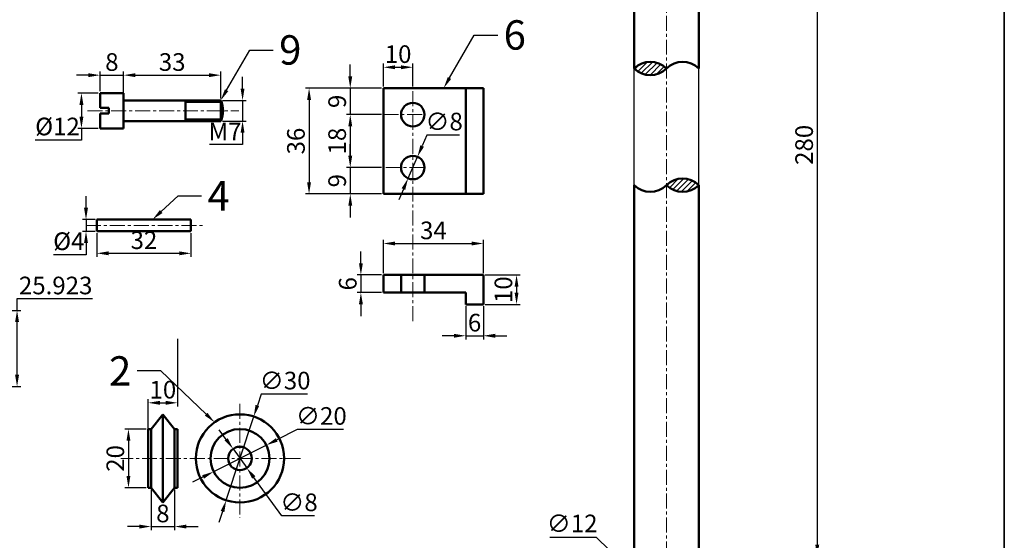
# Model space of a CAD drawing. Units: millimetres. Extents: x 44 to 571, y -292 to 291.
# Tile 3 of 4: x 236 to 571, y -69 to 108. Entities that reach past the tile are written whole.
import ezdxf
from ezdxf import colors
from ezdxf.entities.mleader import LeaderData, LeaderLine
from ezdxf.math import Vec2, Vec3

# ---------------------------------------------------------------- set-up
doc = ezdxf.new("R2010")
doc.units = ezdxf.units.MM
doc.header["$LTSCALE"] = 0.4
doc.linetypes.add('CENTER', pattern=[50.8, 31.75, -6.35, 6.35, -6.35])
for name, color, linetype, lineweight in [('M-CNTR', 1, 'CENTER', 18), ('M-DIMS', 2, 'Continuous', 25), ('M-HATC', 8, 'Continuous', 18), ('M-OUTL', 7, 'Continuous', 50), ('M-TEXT', 3, 'Continuous', 25), ('M-TTLB', 7, 'Continuous', 35)]:
    doc.layers.add(name, color=color, linetype=linetype, lineweight=lineweight)
doc.styles.get("Standard").update_dxf_attribs({"font": 'arial.ttf'})
doc.dimstyles.new('ISO-25', dxfattribs={"dimtxt": 6, "dimasz": 4, "dimexe": 1.25, "dimexo": 0.625, "dimtad": 1, "dimtoh": 1, "dimdec": 0, "dimtxsty": 'Standard', "dimcen": 2.5, "dimadec": 0, "dimazin": 0, "dimtfac": 1, "dimtdec": 0, "dimtmove": 0, "dimatfit": 3, "dimfxl": 1, "dimarcsym": 0})

# ---------------------------------------------------------------- blocks, each defined once
blk = doc.blocks.new('*D37')
at = {"layer": 'Defpoints', "color": 0, "ltscale": 0.4, "transparency": 16777216}
for p in [(271.14, 89.1), (263.14, 83), (271.14, 83)]:
    blk.add_point(p, dxfattribs=at)
at = {"layer": 'M-DIMS', "color": 0, "lineweight": -2, "ltscale": 0.4, "transparency": 16777216}
for p, q in [((259.14, 89.1), (255.14, 89.1)), ((263.14, 83.63), (263.14, 90.35)), ((263.14, 89.1), (271.14, 89.1)), ((271.14, 83.63), (271.14, 90.35)), ((275.14, 89.1), (279.14, 89.1))]:
    blk.add_line(p, q, dxfattribs=at)
at = {"layer": 'M-DIMS', "color": 0, "ltscale": 0.4, "transparency": 16777216}
for points in [[(259.14, 89.77), (259.14, 88.44), (263.14, 89.1)], [(275.14, 89.77), (275.14, 88.44), (271.14, 89.1)]]:
    blk.add_solid(points, dxfattribs=at)
at = {"layer": 'M-DIMS', "color": 0, "ltscale": 0.4, "transparency": 16777216, "insert": (267.14, 92.79), "char_height": 6, "attachment_point": 5}
blk.add_mtext('8', dxfattribs=at)
blk = doc.blocks.new('*D38')
at = {"layer": 'Defpoints', "color": 0, "ltscale": 0.4, "transparency": 16777216}
for p in [(304.14, 89.1), (271.14, 80.5), (304.14, 80.5)]:
    blk.add_point(p, dxfattribs=at)
at = {"layer": 'M-DIMS', "color": 0, "lineweight": -2, "ltscale": 0.4, "transparency": 16777216}
for p, q in [((271.14, 81.13), (271.14, 90.35)), ((275.14, 89.1), (300.14, 89.1)), ((304.14, 81.13), (304.14, 90.35))]:
    blk.add_line(p, q, dxfattribs=at)
at = {"layer": 'M-DIMS', "color": 0, "ltscale": 0.4, "transparency": 16777216}
for points in [[(275.14, 89.77), (275.14, 88.44), (271.14, 89.1)], [(300.14, 89.77), (300.14, 88.44), (304.14, 89.1)]]:
    blk.add_solid(points, dxfattribs=at)
at = {"layer": 'M-DIMS', "color": 0, "ltscale": 0.4, "transparency": 16777216, "insert": (287.64, 92.79), "char_height": 6, "attachment_point": 5}
blk.add_mtext('33', dxfattribs=at)
blk = doc.blocks.new('*D39')
at = {"layer": 'Defpoints', "color": 0, "ltscale": 0.4, "transparency": 16777216}
for p in [(304.14, 80.5), (304.14, 73.5), (311.58, 73.5)]:
    blk.add_point(p, dxfattribs=at)
at = {"layer": 'M-DIMS', "color": 0, "lineweight": -2, "ltscale": 0.4, "transparency": 16777216}
for p, q in [((311.58, 84.5), (311.58, 88.5)), ((304.77, 80.5), (312.83, 80.5)), ((311.58, 80.5), (311.58, 73.5)), ((304.77, 73.5), (312.83, 73.5)), ((311.58, 69.5), (311.58, 65.5)), ((311.58, 65.5), (300.31, 65.5))]:
    blk.add_line(p, q, dxfattribs=at)
at = {"layer": 'M-DIMS', "color": 0, "ltscale": 0.4, "transparency": 16777216}
for points in [[(310.91, 84.5), (312.24, 84.5), (311.58, 80.5)], [(310.91, 69.5), (312.24, 69.5), (311.58, 73.5)]]:
    blk.add_solid(points, dxfattribs=at)
at = {"layer": 'M-DIMS', "color": 0, "ltscale": 0.4, "transparency": 16777216, "insert": (305.63, 69.13), "char_height": 6, "attachment_point": 5}
blk.add_mtext('M7', dxfattribs=at)
blk = doc.blocks.new('*D40')
at = {"layer": 'Defpoints', "color": 0, "ltscale": 0.4, "transparency": 16777216}
for p in [(263.14, 83), (256.8, 71), (263.14, 71)]:
    blk.add_point(p, dxfattribs=at)
at = {"layer": 'M-DIMS', "color": 0, "lineweight": -2, "ltscale": 0.4, "transparency": 16777216}
for p, q in [((262.52, 83), (255.55, 83)), ((256.8, 79), (256.8, 75)), ((262.52, 71), (255.55, 71)), ((256.8, 71), (256.8, 67)), ((256.8, 67), (241.11, 67))]:
    blk.add_line(p, q, dxfattribs=at)
at = {"layer": 'M-DIMS', "color": 0, "ltscale": 0.4, "transparency": 16777216}
for points in [[(256.13, 79), (257.47, 79), (256.8, 83)], [(256.13, 75), (257.47, 75), (256.8, 71)]]:
    blk.add_solid(points, dxfattribs=at)
at = {"layer": 'M-DIMS', "color": 0, "ltscale": 0.4, "transparency": 16777216, "insert": (248.65, 70.86), "char_height": 6, "attachment_point": 5}
blk.add_mtext('%%C12', dxfattribs=at)
blk = doc.blocks.new('*D41')
at = {"layer": 'Defpoints', "color": 0, "ltscale": 0.4, "transparency": 16777216}
for p in [(359.46, 21.12), (351.81, 15.12), (359.46, 15.12)]:
    blk.add_point(p, dxfattribs=at)
at = {"layer": 'M-DIMS', "color": 0, "lineweight": -2, "ltscale": 0.4, "transparency": 16777216}
for p, q in [((351.81, 25.12), (351.81, 29.12)), ((358.83, 21.12), (350.56, 21.12)), ((351.81, 21.12), (351.81, 15.12)), ((358.83, 15.12), (350.56, 15.12)), ((351.81, 11.12), (351.81, 7.12))]:
    blk.add_line(p, q, dxfattribs=at)
at = {"layer": 'M-DIMS', "color": 0, "ltscale": 0.4, "transparency": 16777216}
for points in [[(351.15, 25.12), (352.48, 25.12), (351.81, 21.12)], [(351.15, 11.12), (352.48, 11.12), (351.81, 15.12)]]:
    blk.add_solid(points, dxfattribs=at)
at = {"layer": 'M-DIMS', "color": 0, "ltscale": 0.4, "transparency": 16777216, "insert": (348.12, 18.12), "char_height": 6, "attachment_point": 5, "rotation": 90}
blk.add_mtext('6', dxfattribs=at)
blk = doc.blocks.new('*D42')
at = {"layer": 'Defpoints', "color": 0, "ltscale": 0.4, "transparency": 16777216}
for p in [(393.46, 31.83), (359.46, 21.12), (393.46, 21.12)]:
    blk.add_point(p, dxfattribs=at)
at = {"layer": 'M-DIMS', "color": 0, "lineweight": -2, "ltscale": 0.4, "transparency": 16777216}
for p, q in [((359.46, 21.75), (359.46, 33.08)), ((363.46, 31.83), (389.46, 31.83)), ((393.46, 21.75), (393.46, 33.08))]:
    blk.add_line(p, q, dxfattribs=at)
at = {"layer": 'M-DIMS', "color": 0, "ltscale": 0.4, "transparency": 16777216}
for points in [[(363.46, 32.5), (363.46, 31.16), (359.46, 31.83)], [(389.46, 32.5), (389.46, 31.16), (393.46, 31.83)]]:
    blk.add_solid(points, dxfattribs=at)
at = {"layer": 'M-DIMS', "color": 0, "ltscale": 0.4, "transparency": 16777216, "insert": (376.46, 35.52), "char_height": 6, "attachment_point": 5}
blk.add_mtext('34', dxfattribs=at)
blk = doc.blocks.new('*D43')
at = {"layer": 'Defpoints', "color": 0, "ltscale": 0.4, "transparency": 16777216}
for p in [(387.46, 11.12), (393.46, 11.12), (393.46, 0.44)]:
    blk.add_point(p, dxfattribs=at)
at = {"layer": 'M-DIMS', "color": 0, "lineweight": -2, "ltscale": 0.4, "transparency": 16777216}
for p, q in [((387.46, 10.5), (387.46, -0.81)), ((393.46, 10.5), (393.46, -0.81)), ((383.46, 0.44), (379.46, 0.44)), ((387.46, 0.44), (393.46, 0.44)), ((397.46, 0.44), (401.46, 0.44))]:
    blk.add_line(p, q, dxfattribs=at)
at = {"layer": 'M-DIMS', "color": 0, "ltscale": 0.4, "transparency": 16777216}
for points in [[(383.46, 1.1), (383.46, -0.23), (387.46, 0.44)], [(397.46, 1.1), (397.46, -0.23), (393.46, 0.44)]]:
    blk.add_solid(points, dxfattribs=at)
at = {"layer": 'M-DIMS', "color": 0, "ltscale": 0.4, "transparency": 16777216, "insert": (390.46, 4.12), "char_height": 6, "attachment_point": 5}
blk.add_mtext('6', dxfattribs=at)
blk = doc.blocks.new('*D44')
at = {"layer": 'Defpoints', "color": 0, "ltscale": 0.4, "transparency": 16777216}
for p in [(393.46, 21.12), (393.46, 11.12), (404.73, 11.12)]:
    blk.add_point(p, dxfattribs=at)
at = {"layer": 'M-DIMS', "color": 0, "lineweight": -2, "ltscale": 0.4, "transparency": 16777216}
for p, q in [((394.08, 21.12), (405.98, 21.12)), ((404.73, 17.12), (404.73, 15.12)), ((394.08, 11.12), (405.98, 11.12))]:
    blk.add_line(p, q, dxfattribs=at)
at = {"layer": 'M-DIMS', "color": 0, "ltscale": 0.4, "transparency": 16777216}
for points in [[(404.06, 17.12), (405.4, 17.12), (404.73, 21.12)], [(404.06, 15.12), (405.4, 15.12), (404.73, 11.12)]]:
    blk.add_solid(points, dxfattribs=at)
at = {"layer": 'M-DIMS', "color": 0, "ltscale": 0.4, "transparency": 16777216, "insert": (401.04, 16.12), "char_height": 6, "attachment_point": 5, "rotation": 90}
blk.add_mtext('10', dxfattribs=at)
blk = doc.blocks.new('*D45')
at = {"layer": 'Defpoints', "color": 0, "ltscale": 0.4, "transparency": 16777216}
for p in [(359.46, 84.68), (348.19, 75.68), (359.46, 75.68)]:
    blk.add_point(p, dxfattribs=at)
at = {"layer": 'M-DIMS', "color": 0, "lineweight": -2, "ltscale": 0.4, "transparency": 16777216}
for p, q in [((348.19, 88.68), (348.19, 92.68)), ((358.83, 84.68), (346.94, 84.68)), ((348.19, 84.68), (348.19, 75.68)), ((358.83, 75.68), (346.94, 75.68)), ((348.19, 71.68), (348.19, 67.68))]:
    blk.add_line(p, q, dxfattribs=at)
at = {"layer": 'M-DIMS', "color": 0, "ltscale": 0.4, "transparency": 16777216}
for points in [[(347.53, 88.68), (348.86, 88.68), (348.19, 84.68)], [(347.53, 71.68), (348.86, 71.68), (348.19, 75.68)]]:
    blk.add_solid(points, dxfattribs=at)
at = {"layer": 'M-DIMS', "color": 0, "ltscale": 0.4, "transparency": 16777216, "insert": (344.51, 80.18), "char_height": 6, "attachment_point": 5, "rotation": 90}
blk.add_mtext('9', dxfattribs=at)
blk = doc.blocks.new('*D46')
at = {"layer": 'Defpoints', "color": 0, "ltscale": 0.4, "transparency": 16777216}
for p in [(359.46, 75.68), (348.19, 57.68), (359.46, 57.68)]:
    blk.add_point(p, dxfattribs=at)
at = {"layer": 'M-DIMS', "color": 0, "lineweight": -2, "ltscale": 0.4, "transparency": 16777216}
for p, q in [((358.83, 75.68), (346.94, 75.68)), ((348.19, 71.68), (348.19, 61.68)), ((358.83, 57.68), (346.94, 57.68))]:
    blk.add_line(p, q, dxfattribs=at)
at = {"layer": 'M-DIMS', "color": 0, "ltscale": 0.4, "transparency": 16777216}
for points in [[(347.53, 71.68), (348.86, 71.68), (348.19, 75.68)], [(347.53, 61.68), (348.86, 61.68), (348.19, 57.68)]]:
    blk.add_solid(points, dxfattribs=at)
at = {"layer": 'M-DIMS', "color": 0, "ltscale": 0.4, "transparency": 16777216, "insert": (344.51, 66.68), "char_height": 6, "attachment_point": 5, "rotation": 90}
blk.add_mtext('18', dxfattribs=at)
blk = doc.blocks.new('*D47')
at = {"layer": 'Defpoints', "color": 0, "ltscale": 0.4, "transparency": 16777216}
for p in [(359.46, 57.68), (348.19, 48.68), (359.46, 48.68)]:
    blk.add_point(p, dxfattribs=at)
at = {"layer": 'M-DIMS', "color": 0, "lineweight": -2, "ltscale": 0.4, "transparency": 16777216}
for p, q in [((348.19, 61.68), (348.19, 65.68)), ((358.83, 57.68), (346.94, 57.68)), ((348.19, 57.68), (348.19, 48.68)), ((358.83, 48.68), (346.94, 48.68)), ((348.19, 44.68), (348.19, 40.68))]:
    blk.add_line(p, q, dxfattribs=at)
at = {"layer": 'M-DIMS', "color": 0, "ltscale": 0.4, "transparency": 16777216}
for points in [[(347.53, 61.68), (348.86, 61.68), (348.19, 57.68)], [(347.53, 44.68), (348.86, 44.68), (348.19, 48.68)]]:
    blk.add_solid(points, dxfattribs=at)
at = {"layer": 'M-DIMS', "color": 0, "ltscale": 0.4, "transparency": 16777216, "insert": (344.51, 53.18), "char_height": 6, "attachment_point": 5, "rotation": 90}
blk.add_mtext('9', dxfattribs=at)
blk = doc.blocks.new('*D48')
at = {"layer": 'Defpoints', "color": 0, "ltscale": 0.4, "transparency": 16777216}
for p in [(359.46, 84.68), (334.19, 48.68), (359.46, 48.68)]:
    blk.add_point(p, dxfattribs=at)
at = {"layer": 'M-DIMS', "color": 0, "lineweight": -2, "ltscale": 0.4, "transparency": 16777216}
for p, q in [((358.83, 84.68), (332.94, 84.68)), ((334.19, 80.68), (334.19, 52.68)), ((358.83, 48.68), (332.94, 48.68))]:
    blk.add_line(p, q, dxfattribs=at)
at = {"layer": 'M-DIMS', "color": 0, "ltscale": 0.4, "transparency": 16777216}
for points in [[(333.52, 80.68), (334.85, 80.68), (334.19, 84.68)], [(333.52, 52.68), (334.85, 52.68), (334.19, 48.68)]]:
    blk.add_solid(points, dxfattribs=at)
at = {"layer": 'M-DIMS', "color": 0, "ltscale": 0.4, "transparency": 16777216, "insert": (330.5, 66.68), "char_height": 6, "attachment_point": 5, "rotation": 90}
blk.add_mtext('36', dxfattribs=at)
blk = doc.blocks.new('*D49')
at = {"layer": 'Defpoints', "color": 0, "ltscale": 0.4, "transparency": 16777216}
for p in [(369.46, 91.79), (359.46, 84.68), (369.46, 84.68)]:
    blk.add_point(p, dxfattribs=at)
at = {"layer": 'M-DIMS', "color": 0, "lineweight": -2, "ltscale": 0.4, "transparency": 16777216}
for p, q in [((359.46, 85.3), (359.46, 93.04)), ((363.46, 91.79), (365.46, 91.79)), ((369.46, 85.3), (369.46, 93.04))]:
    blk.add_line(p, q, dxfattribs=at)
at = {"layer": 'M-DIMS', "color": 0, "ltscale": 0.4, "transparency": 16777216}
for points in [[(363.46, 92.45), (363.46, 91.12), (359.46, 91.79)], [(365.46, 92.45), (365.46, 91.12), (369.46, 91.79)]]:
    blk.add_solid(points, dxfattribs=at)
at = {"layer": 'M-DIMS', "color": 0, "ltscale": 0.4, "transparency": 16777216, "insert": (364.46, 95.48), "char_height": 6, "attachment_point": 5}
blk.add_mtext('10', dxfattribs=at)
blk = doc.blocks.new('*D50')
at = {"layer": 'Defpoints', "color": 0, "ltscale": 0.4, "transparency": 16777216}
for p in [(371.05, 61.35), (367.86, 54.01)]:
    blk.add_point(p, dxfattribs=at)
at = {"layer": 'M-DIMS', "color": 0, "lineweight": -2, "ltscale": 0.4, "transparency": 16777216}
for p, q in [((374.24, 68.68), (372.65, 65.01)), ((385.34, 68.68), (374.24, 68.68)), ((367.86, 54.01), (371.05, 61.35)), ((366.27, 50.34), (364.68, 46.67))]:
    blk.add_line(p, q, dxfattribs=at)
at = {"layer": 'M-DIMS', "color": 0, "ltscale": 0.4, "transparency": 16777216}
for points in [[(372.03, 65.28), (373.26, 64.75), (371.05, 61.35)], [(365.66, 50.61), (366.88, 50.07), (367.86, 54.01)]]:
    blk.add_solid(points, dxfattribs=at)
at = {"layer": 'M-DIMS', "color": 0, "ltscale": 0.4, "transparency": 16777216, "insert": (380.1, 72.54), "char_height": 6, "attachment_point": 5}
blk.add_mtext('∅8', dxfattribs=at)
blk = doc.blocks.new('*D51')
at = {"layer": 'Defpoints', "color": 0, "ltscale": 0.4, "transparency": 16777216}
for p in [(262.04, 39.97), (258.35, 35.97), (262.04, 35.97)]:
    blk.add_point(p, dxfattribs=at)
at = {"layer": 'M-DIMS', "color": 0, "lineweight": -2, "ltscale": 0.4, "transparency": 16777216}
for p, q in [((258.35, 43.97), (258.35, 47.97)), ((261.42, 39.97), (257.1, 39.97)), ((258.35, 39.97), (258.35, 35.97)), ((261.42, 35.97), (257.1, 35.97)), ((258.35, 31.97), (258.35, 27.97)), ((258.35, 27.97), (247.28, 27.97))]:
    blk.add_line(p, q, dxfattribs=at)
at = {"layer": 'M-DIMS', "color": 0, "ltscale": 0.4, "transparency": 16777216}
for points in [[(257.68, 43.97), (259.01, 43.97), (258.35, 39.97)], [(257.68, 31.97), (259.01, 31.97), (258.35, 35.97)]]:
    blk.add_solid(points, dxfattribs=at)
at = {"layer": 'M-DIMS', "color": 0, "ltscale": 0.4, "transparency": 16777216, "insert": (252.5, 31.83), "char_height": 6, "attachment_point": 5}
blk.add_mtext('%%C4', dxfattribs=at)
blk = doc.blocks.new('*D52')
at = {"layer": 'Defpoints', "color": 0, "ltscale": 0.4, "transparency": 16777216}
for p in [(262.04, 35.97), (294.04, 35.97), (294.04, 28.49)]:
    blk.add_point(p, dxfattribs=at)
at = {"layer": 'M-DIMS', "color": 0, "lineweight": -2, "ltscale": 0.4, "transparency": 16777216}
for p, q in [((262.04, 35.35), (262.04, 27.24)), ((294.04, 35.35), (294.04, 27.24)), ((266.04, 28.49), (290.04, 28.49))]:
    blk.add_line(p, q, dxfattribs=at)
at = {"layer": 'M-DIMS', "color": 0, "ltscale": 0.4, "transparency": 16777216}
for points in [[(266.04, 29.16), (266.04, 27.82), (262.04, 28.49)], [(290.04, 29.16), (290.04, 27.82), (294.04, 28.49)]]:
    blk.add_solid(points, dxfattribs=at)
at = {"layer": 'M-DIMS', "color": 0, "ltscale": 0.4, "transparency": 16777216, "insert": (278.04, 32.18), "char_height": 6, "attachment_point": 5}
blk.add_mtext('32', dxfattribs=at)
blk = doc.blocks.new('*D53')
at = {"layer": 'Defpoints', "color": 0, "ltscale": 0.4, "transparency": 16777216}
for p in [(466.7, 205.39), (466.7, -74.61), (506.97, -74.61)]:
    blk.add_point(p, dxfattribs=at)
at = {"layer": 'M-DIMS', "color": 0, "lineweight": -2, "ltscale": 0.4, "transparency": 16777216}
for p, q in [((467.32, 205.39), (508.22, 205.39)), ((506.97, 201.39), (506.97, -70.61)), ((467.32, -74.61), (508.22, -74.61))]:
    blk.add_line(p, q, dxfattribs=at)
at = {"layer": 'M-DIMS', "color": 0, "ltscale": 0.4, "transparency": 16777216}
for points in [[(506.3, 201.39), (507.64, 201.39), (506.97, 205.39)], [(506.3, -70.61), (507.64, -70.61), (506.97, -74.61)]]:
    blk.add_solid(points, dxfattribs=at)
at = {"layer": 'M-DIMS', "color": 0, "ltscale": 0.4, "transparency": 16777216, "insert": (503.28, 65.39), "char_height": 6, "attachment_point": 5, "rotation": 90}
blk.add_mtext('280', dxfattribs=at)
blk = doc.blocks.new('*D63')
at = {"layer": 'Defpoints', "color": 0, "ltscale": 0.4, "transparency": 16777216}
for p in [(451.4, -87.13), (460, -95.5)]:
    blk.add_point(p, dxfattribs=at)
at = {"layer": 'M-DIMS', "color": 0, "lineweight": -2, "ltscale": 0.4, "transparency": 16777216}
for p, q in [((416.09, -68.05), (431.77, -68.05)), ((431.77, -68.05), (448.53, -84.34)), ((460, -95.5), (451.4, -87.13)), ((462.86, -98.29), (465.73, -101.08))]:
    blk.add_line(p, q, dxfattribs=at)
at = {"layer": 'M-DIMS', "color": 0, "ltscale": 0.4, "transparency": 16777216}
for points in [[(448.99, -83.86), (448.06, -84.82), (451.4, -87.13)], [(463.33, -97.81), (462.4, -98.76), (460, -95.5)]]:
    blk.add_solid(points, dxfattribs=at)
at = {"layer": 'M-DIMS', "color": 0, "ltscale": 0.4, "transparency": 16777216, "insert": (423.62, -64.19), "char_height": 6, "attachment_point": 5}
blk.add_mtext('∅12', dxfattribs=at)
blk = doc.blocks.new('*D65')
at = {"layer": 'Defpoints', "color": 0, "ltscale": 0.4, "transparency": 16777216}
for p in [(279.48, -31.29), (272.78, -51.29), (279.48, -51.29)]:
    blk.add_point(p, dxfattribs=at)
at = {"layer": 'M-DIMS', "color": 0, "lineweight": -2, "ltscale": 0.4, "transparency": 16777216}
for p, q in [((278.85, -31.29), (271.53, -31.29)), ((272.78, -35.29), (272.78, -47.29)), ((278.85, -51.29), (271.53, -51.29))]:
    blk.add_line(p, q, dxfattribs=at)
at = {"layer": 'M-DIMS', "color": 0, "ltscale": 0.4, "transparency": 16777216}
for points in [[(272.11, -35.29), (273.44, -35.29), (272.78, -31.29)], [(272.11, -47.29), (273.44, -47.29), (272.78, -51.29)]]:
    blk.add_solid(points, dxfattribs=at)
at = {"layer": 'M-DIMS', "color": 0, "ltscale": 0.4, "transparency": 16777216, "insert": (269.09, -41.29), "char_height": 6, "attachment_point": 5, "rotation": 90}
blk.add_mtext('20', dxfattribs=at)
blk = doc.blocks.new('*D66')
at = {"layer": 'Defpoints', "color": 0, "ltscale": 0.4, "transparency": 16777216}
for p in [(280.48, -51.29), (288.48, -51.29), (288.48, -64.47)]:
    blk.add_point(p, dxfattribs=at)
at = {"layer": 'M-DIMS', "color": 0, "lineweight": -2, "ltscale": 0.4, "transparency": 16777216}
for p, q in [((280.48, -51.91), (280.48, -65.72)), ((288.48, -51.91), (288.48, -65.72)), ((276.48, -64.47), (272.48, -64.47)), ((280.48, -64.47), (288.48, -64.47)), ((292.48, -64.47), (296.48, -64.47))]:
    blk.add_line(p, q, dxfattribs=at)
at = {"layer": 'M-DIMS', "color": 0, "ltscale": 0.4, "transparency": 16777216}
for points in [[(276.48, -63.81), (276.48, -65.14), (280.48, -64.47)], [(292.48, -63.81), (292.48, -65.14), (288.48, -64.47)]]:
    blk.add_solid(points, dxfattribs=at)
at = {"layer": 'M-DIMS', "color": 0, "ltscale": 0.4, "transparency": 16777216, "insert": (284.48, -60.79), "char_height": 6, "attachment_point": 5}
blk.add_mtext('8', dxfattribs=at)
blk = doc.blocks.new('*D67')
at = {"layer": 'Defpoints', "color": 0, "ltscale": 0.4, "transparency": 16777216}
for p in [(289.48, 0), (289.48, -22.37), (279.48, -51.29)]:
    blk.add_point(p, dxfattribs=at)
at = {"layer": 'M-DIMS', "color": 0, "lineweight": -2, "ltscale": 0.4, "transparency": 16777216}
for p, q in [((289.48, -0.62), (289.48, -23.62)), ((279.48, -50.66), (279.48, -21.12)), ((283.48, -22.37), (285.48, -22.37))]:
    blk.add_line(p, q, dxfattribs=at)
at = {"layer": 'M-DIMS', "color": 0, "ltscale": 0.4, "transparency": 16777216}
for points in [[(283.48, -21.7), (283.48, -23.03), (279.48, -22.37)], [(285.48, -21.7), (285.48, -23.03), (289.48, -22.37)]]:
    blk.add_solid(points, dxfattribs=at)
at = {"layer": 'M-DIMS', "color": 0, "ltscale": 0.4, "transparency": 16777216, "insert": (284.48, -18.68), "char_height": 6, "attachment_point": 5}
blk.add_mtext('10', dxfattribs=at)
blk = doc.blocks.new('*D68')
at = {"layer": 'Defpoints', "color": 0, "ltscale": 0.4, "transparency": 16777216}
for p in [(308.34, -38.05), (313.04, -44.53)]:
    blk.add_point(p, dxfattribs=at)
at = {"layer": 'M-DIMS', "color": 0, "lineweight": -2, "ltscale": 0.4, "transparency": 16777216}
for p, q in [((305.99, -34.82), (303.64, -31.58)), ((308.34, -38.05), (313.04, -44.53)), ((324.9, -60.85), (315.39, -47.76)), ((336, -60.85), (324.9, -60.85))]:
    blk.add_line(p, q, dxfattribs=at)
at = {"layer": 'M-DIMS', "color": 0, "ltscale": 0.4, "transparency": 16777216}
for points in [[(306.53, -34.42), (305.45, -35.21), (308.34, -38.05)], [(315.93, -47.37), (314.85, -48.15), (313.04, -44.53)]]:
    blk.add_solid(points, dxfattribs=at)
at = {"layer": 'M-DIMS', "color": 0, "ltscale": 0.4, "transparency": 16777216, "insert": (330.76, -57), "char_height": 6, "attachment_point": 5}
blk.add_mtext('∅8', dxfattribs=at)
blk = doc.blocks.new('*D69')
at = {"layer": 'Defpoints', "color": 0, "ltscale": 0.4, "transparency": 16777216}
for p in [(319.62, -36.79), (301.76, -45.78)]:
    blk.add_point(p, dxfattribs=at)
at = {"layer": 'M-DIMS', "color": 0, "lineweight": -2, "ltscale": 0.4, "transparency": 16777216}
for p, q in [((330.19, -31.48), (323.2, -35)), ((345.91, -31.48), (330.19, -31.48)), ((301.76, -45.78), (319.62, -36.79)), ((298.18, -47.58), (294.61, -49.38))]:
    blk.add_line(p, q, dxfattribs=at)
at = {"layer": 'M-DIMS', "color": 0, "ltscale": 0.4, "transparency": 16777216}
for points in [[(322.9, -34.4), (323.5, -35.59), (319.62, -36.79)], [(297.88, -46.99), (298.48, -48.18), (301.76, -45.78)]]:
    blk.add_solid(points, dxfattribs=at)
at = {"layer": 'M-DIMS', "color": 0, "ltscale": 0.4, "transparency": 16777216, "insert": (338.36, -27.62), "char_height": 6, "attachment_point": 5}
blk.add_mtext('∅20', dxfattribs=at)
blk = doc.blocks.new('*D70')
at = {"layer": 'Defpoints', "color": 0, "ltscale": 0.4, "transparency": 16777216}
for p in [(315.37, -27.04), (306.01, -55.54)]:
    blk.add_point(p, dxfattribs=at)
at = {"layer": 'M-DIMS', "color": 0, "lineweight": -2, "ltscale": 0.4, "transparency": 16777216}
for p, q in [((317.87, -19.44), (316.62, -23.24)), ((333.6, -19.44), (317.87, -19.44)), ((306.01, -55.54), (315.37, -27.04)), ((304.76, -59.34), (303.51, -63.14))]:
    blk.add_line(p, q, dxfattribs=at)
at = {"layer": 'M-DIMS', "color": 0, "ltscale": 0.4, "transparency": 16777216}
for points in [[(315.99, -23.03), (317.25, -23.45), (315.37, -27.04)], [(304.13, -59.13), (305.39, -59.55), (306.01, -55.54)]]:
    blk.add_solid(points, dxfattribs=at)
at = {"layer": 'M-DIMS', "color": 0, "ltscale": 0.4, "transparency": 16777216, "insert": (326.05, -15.58), "char_height": 6, "attachment_point": 5}
blk.add_mtext('∅30', dxfattribs=at)
blk = doc.blocks.new('*D75')
at = {"layer": 'Defpoints', "color": 0, "ltscale": 0.4, "transparency": 16777216}
for p in [(153.17, 9.08), (234.9, 9.08), (175.17, -16.85)]:
    blk.add_point(p, dxfattribs=at)
at = {"layer": 'M-DIMS', "color": 0, "lineweight": -2, "ltscale": 0.4, "transparency": 16777216}
for p, q in [((234.9, 9.08), (234.9, 13.08)), ((234.9, 13.08), (260.54, 13.08)), ((153.79, 9.08), (236.15, 9.08)), ((234.9, -12.85), (234.9, 5.08)), ((175.79, -16.85), (236.15, -16.85))]:
    blk.add_line(p, q, dxfattribs=at)
at = {"layer": 'M-DIMS', "color": 0, "ltscale": 0.4, "transparency": 16777216}
for points in [[(234.23, 5.08), (235.57, 5.08), (234.9, 9.08)], [(234.23, -12.85), (235.57, -12.85), (234.9, -16.85)]]:
    blk.add_solid(points, dxfattribs=at)
at = {"layer": 'M-DIMS', "color": 0, "ltscale": 0.4, "transparency": 16777216, "insert": (248.03, 16.77), "char_height": 6, "attachment_point": 5}
blk.add_mtext('25.923', dxfattribs=at)
blk = doc.blocks.new('*D77')
at = {"layer": 'Defpoints', "color": 0, "ltscale": 0.4, "transparency": 16777216}
for p in [(466.7, 250.52), (444.7, -228.61), (466.7, -228.61)]:
    blk.add_point(p, dxfattribs=at)
at = {"layer": 'M-DIMS', "color": 0, "lineweight": -2, "ltscale": 0.4, "transparency": 16777216}
for p, q in [((444.7, -227.99), (444.7, 251.77)), ((466.7, -227.99), (466.7, 251.77)), ((448.7, 250.52), (462.7, 250.52))]:
    blk.add_line(p, q, dxfattribs=at)
at = {"layer": 'M-DIMS', "color": 0, "ltscale": 0.4, "transparency": 16777216}
for points in [[(448.7, 251.19), (448.7, 249.85), (444.7, 250.52)], [(462.7, 251.19), (462.7, 249.85), (466.7, 250.52)]]:
    blk.add_solid(points, dxfattribs=at)
at = {"layer": 'M-DIMS', "color": 0, "ltscale": 0.4, "transparency": 16777216, "insert": (455.7, 254.16), "char_height": 6, "attachment_point": 5}
blk.add_mtext('22', dxfattribs=at)

msp = doc.modelspace()

# ---------------------------------------------------------------- hatches: boundary and pattern name
at = {"layer": 'M-HATC', "ltscale": 0.4}
h = msp.add_hatch(dxfattribs=at)
h.set_pattern_fill('ANSI31', color=256, scale=0.4)
h.paths.add_polyline_path([(466.6963, 51.668), (466.6963, 51.668, 0.41365763), (455.6963, 51.668, 0.41365763)])
h.paths.add_polyline_path([(444.6963, 91.3959, 0.41365763), (455.6963, 91.3959, 0.41365763)])
h.paths.add_polyline_path([(171.2864, 238.6681), (441.8676, 238.6681), (441.8676, 283.6094), (171.2864, 283.6094)], flags=9)

# ---------------------------------------------------------------- linework, layer by layer
at = {"layer": 'M-CNTR', "ltscale": 0.4}
for p, q in [((455.6963, -74.6115), (455.6963, 225.3706)), ((369.4572, 5.4252), (369.4572, 84.6772)), ((258.825, 77.0036), (310.3561, 77.0036)), ((359.4572, 75.6772), (373.4572, 75.6772)), ((373.4572, 57.6772), (359.4572, 57.6772)), ((258.3451, 37.9741), (298.238, 37.9741)), ((310.6899, -22.7225), (310.6899, -61.3339)), ((331.2401, -41.2891), (270.2286, -41.2891))]:
    msp.add_line(p, q, dxfattribs=at)
at = {"layer": 'M-OUTL', "ltscale": 0.4}
for p, q in [((444.6963, 91.3959), (444.6963, 205.3885)), ((466.6963, 205.3885), (466.6963, 91.3959)), ((359.4572, 48.6772), (359.4572, 84.6772)), ((359.4572, 84.6772), (393.4572, 84.6772)), ((387.4572, 84.6772), (387.4572, 48.6772)), ((393.4572, 84.6772), (393.4572, 48.6772)), ((263.1449, 83.0036), (271.1449, 83.0036)), ((263.1449, 78.0036), (263.1449, 83.0036)), ((271.1449, 83.0036), (271.1449, 71.0036)), ((271.1449, 80.5036), (304.1449, 80.5036)), ((292.1449, 80.5036), (292.1449, 73.5036)), ((304.1449, 80.5036), (304.1449, 73.5036)), ((263.1449, 78.0036), (266.1449, 78.0036)), ((266.1449, 78.0036), (266.1449, 76.0036)), ((292.1449, 80.0036), (304.1449, 80.0036)), ((263.1449, 71.0036), (263.1449, 76.0036)), ((266.1449, 76.0036), (263.1449, 76.0036)), ((292.1449, 74.0036), (304.1449, 74.0036)), ((271.1449, 71.0036), (263.1449, 71.0036)), ((271.1449, 73.5036), (304.1449, 73.5036)), ((444.6963, -74.6115), (444.6963, 51.668)), ((466.6963, 51.668), (466.6963, -74.6115)), ((393.4572, 48.6772), (359.4572, 48.6772)), ((262.041, 39.9741), (294.041, 39.9741)), ((262.041, 35.9741), (262.041, 39.9741)), ((294.041, 39.9741), (294.041, 35.9741)), ((294.041, 35.9741), (262.041, 35.9741)), ((393.4572, 21.1232), (359.4572, 21.1232)), ((359.4572, 21.1232), (359.4572, 15.1232)), ((365.4572, 21.1232), (365.4572, 15.1232)), ((373.4572, 21.1232), (373.4572, 15.1232)), ((393.4572, 11.1232), (393.4572, 21.1232)), ((359.4572, 15.1232), (387.4572, 15.1232)), ((387.4572, 15.1232), (387.4572, 11.1232)), ((387.4572, 11.1232), (393.4572, 11.1232)), ((284.4769, -26.2891), (280.4769, -31.2891)), ((284.4769, -26.2891), (284.4769, -56.2891)), ((284.4769, -26.2891), (288.4769, -31.2891)), ((279.4769, -31.2891), (279.4769, -51.2891)), ((279.4769, -31.2891), (280.4769, -31.2891)), ((280.4769, -31.2891), (280.4769, -51.2891)), ((288.4769, -31.2891), (288.4769, -51.2891)), ((288.4769, -31.2891), (289.4769, -31.2891)), ((289.4769, -31.2891), (289.4769, -51.2891)), ((279.4769, -51.2891), (280.4769, -51.2891)), ((280.4769, -51.2891), (284.4769, -56.2891)), ((284.4769, -56.2891), (288.4769, -51.2891)), ((289.4769, -51.2891), (288.4769, -51.2891))]:
    msp.add_line(p, q, dxfattribs=at)
for centre, radius in [((369.4572, 75.6772), 4), ((369.4572, 57.6772), 4), ((310.6899, -41.2891), 15), ((310.6899, -41.2891), 10), ((310.6899, -41.2891), 4)]:
    msp.add_circle(centre, radius, dxfattribs=at)
for centre, radius, start, end in [((450.1963, 85.8854), 7.7856, 45.054386, 134.945614), ((450.1963, 96.9063), 7.7856, 225.054386, 314.945614), ((461.1963, 85.8854), 7.7856, 45.054386, 134.945614), ((296.7376, 77.0036), 8.1925, 334.708824, 25.291176), ((461.1963, 46.1576), 7.7856, 45.054386, 134.945614), ((450.1963, 57.1785), 7.7856, 225.054386, 314.945614), ((450.1963, 46.1576), 7.7856, 45.054386, 45.054391), ((461.1963, 57.1785), 7.7856, 225.054386, 314.945614)]:
    msp.add_arc(centre, radius, start, end, dxfattribs=at)
at = {"layer": 'M-TTLB', "ltscale": 0.4}
msp.add_lwpolyline([(44.037, 291.1069), (570.566, 291.1069), (570.566, -292.0762), (44.037, -292.0762)], close=True, dxfattribs=at)

# ---------------------------------------------------------------- dimensions: what is measured, and where the dimension line sits
at = {"layer": 'M-DIMS', "ltscale": 0.4}
for base, p1, p2, override, picture, middle in [((466.6963, 250.5206), (444.6963, -228.6115), (466.6963, -228.6115), {"dimdec": 0, "dimlfac": 1, "dimrnd": 0, "dimzin": 0, "dimdsep": 46, "dimlunit": 2}, '*D77', (455.6963, 254.1579)), ((369.4572, 91.7867), (359.4572, 84.6772), (369.4572, 84.6772), {"dimclrd": 0, "dimclre": 0, "dimclrt": 0}, '*D49', (364.4572, 95.4751)), ((271.1449, 89.1018), (263.1449, 83.0036), (271.1449, 83.0036), {"dimclrd": 0, "dimclre": 0, "dimclrt": 0}, '*D37', (267.1449, 92.7902)), ((304.1449, 89.1018), (271.1449, 80.5036), (304.1449, 80.5036), {"dimclrd": 0, "dimclre": 0, "dimclrt": 0}, '*D38', (287.6449, 92.7922)), ((393.4572, 31.8302), (359.4572, 21.1232), (393.4572, 21.1232), {"dimclrd": 0, "dimclre": 0, "dimclrt": 0}, '*D42', (376.4572, 35.5206)), ((294.041, 28.4884), (262.041, 35.9741), (294.041, 35.9741), {"dimclrd": 0, "dimclre": 0, "dimclrt": 0}, '*D52', (278.041, 32.1788)), ((393.4572, 0.4362), (387.4572, 11.1232), (393.4572, 11.1232), {"dimclrd": 0, "dimclre": 0, "dimclrt": 0}, '*D43', (390.4572, 4.1246)), ((289.4769, -22.3662), (279.4769, -51.2891), (289.4769, 0), {"dimclrd": 0, "dimclre": 0, "dimclrt": 0}, '*D67', (284.4769, -18.6778)), ((288.4769, -64.4748), (280.4769, -51.2891), (288.4769, -51.2891), {"dimclrd": 0, "dimclre": 0, "dimclrt": 0}, '*D66', (284.4769, -60.7863))]:
    dim = msp.add_linear_dim(base=base, p1=p1, p2=p2, dimstyle='ISO-25', override=override, dxfattribs=at)
    dim.commit()
    dim.dimension.update_dxf_attribs({"geometry": picture, "text_midpoint": middle})
for base, p1, p2, override, picture, middle in [((506.9684, -74.6115), (466.6963, 205.3885), (466.6963, -74.6115), {"dimclrd": 0, "dimclre": 0, "dimclrt": 0}, '*D53', (503.2799, 65.3885)), ((348.1946, 75.6772), (359.4572, 84.6772), (359.4572, 75.6772), {"dimclrd": 0, "dimclre": 0, "dimclrt": 0}, '*D45', (344.5062, 80.1772)), ((334.1862, 48.6772), (359.4572, 84.6772), (359.4572, 48.6772), {"dimclrd": 0, "dimclre": 0, "dimclrt": 0}, '*D48', (330.4957, 66.6772)), ((348.1946, 57.6772), (359.4572, 75.6772), (359.4572, 57.6772), {"dimclrd": 0, "dimclre": 0, "dimclrt": 0}, '*D46', (344.5062, 66.6772)), ((348.1946, 48.6772), (359.4572, 57.6772), (359.4572, 48.6772), {"dimclrd": 0, "dimclre": 0, "dimclrt": 0}, '*D47', (344.5062, 53.1772)), ((351.8118, 15.1232), (359.4572, 21.1232), (359.4572, 15.1232), {"dimclrd": 0, "dimclre": 0, "dimclrt": 0}, '*D41', (348.1234, 18.1232)), ((234.8992, 9.0761), (175.1682, -16.8469), (153.1682, 9.0761), {"dimdec": 3, "dimlfac": 1, "dimrnd": 0, "dimzin": 0, "dimdsep": 46, "dimlunit": 2}, '*D75', (248.0297, 16.7665)), ((404.729, 11.1232), (393.4572, 21.1232), (393.4572, 11.1232), {"dimclrd": 0, "dimclre": 0, "dimclrt": 0}, '*D44', (401.0405, 16.1232)), ((272.7766, -51.2891), (279.4769, -31.2891), (279.4769, -51.2891), {"dimclrd": 0, "dimclre": 0, "dimclrt": 0}, '*D65', (269.0881, -41.2891))]:
    dim = msp.add_linear_dim(base=base, p1=p1, p2=p2, angle=90, dimstyle='ISO-25', override=override, dxfattribs=at)
    dim.commit()
    dim.dimension.update_dxf_attribs({"geometry": picture, "text_midpoint": middle})
for base, p1, p2, text, picture, middle in [((311.5762, 73.5036), (304.1449, 80.5036), (304.1449, 73.5036), 'M<>', '*D39', (305.6306, 69.1286)), ((256.8013, 71.0036), (263.1449, 83.0036), (263.1449, 71.0036), '%%C<>', '*D40', (248.6457, 70.8598)), ((258.3451, 35.9741), (262.041, 39.9741), (262.041, 35.9741), '%%C<>', '*D51', (252.5018, 31.8304))]:
    dim = msp.add_linear_dim(base=base, p1=p1, p2=p2, angle=90, text=text, dimstyle='ISO-25', override={"dimclrd": 0, "dimclre": 0, "dimclrt": 0}, dxfattribs=at)
    dim.commit()
    dim.dimension.update_dxf_attribs({"geometry": picture, "text_midpoint": middle})
for p1, p2, picture, middle in [((367.8631, 54.0085), (371.0512, 61.3458), '*D50', (380.101, 72.5394)), ((306.0072, -55.5394), (315.3726, -27.0387), '*D70', (326.0462, -15.5823))]:
    dim = msp.add_diameter_dim_2p(p1=p1, p2=p2, dimstyle='ISO-25', override={"dimclrd": 0, "dimclre": 0, "dimclrt": 0}, dxfattribs=at)
    dim.commit()
    dim.dimension.update_dxf_attribs({"geometry": picture, "text_midpoint": middle})
for p1, p2, picture, middle in [((301.7574, -45.7847), (319.6224, -36.7934), '*D69', (338.3613, -31.4773)), ((308.3392, -38.0527), (313.0405, -44.5255), '*D68', (330.7617, -60.8539)), ((459.9974, -95.4982), (451.3952, -87.1315), '*D63', (423.6163, -68.0455))]:
    dim = msp.add_diameter_dim_2p(p1=p1, p2=p2, dimstyle='ISO-25', override={"dimclrd": 0, "dimclre": 0, "dimclrt": 0}, dxfattribs=at)
    dim.commit()
    dim.dimension.update_dxf_attribs({"geometry": picture, "text_midpoint": middle, "dimtype": 163})

# ---------------------------------------------------------------- leaders
at = {"layer": 'M-TEXT', "ltscale": 0.4}
ml = msp.add_multileader_mtext('Standard', dxfattribs=at)
ml.set_content('6', color=256)
ml.set_leader_properties()
ml.build(insert=Vec2(0, 0))
ctx = ml.context
ctx.base_point, ctx.char_height, ctx.plane_origin = Vec3(398.341, 102.6974), 10, Vec3(379.937, 84.6772)
notes = []
notes.append((ctx, [(0, (1, 1, 0), (390.341, 102.6974), (1, 0), 8, [(0, [(379.937, 84.6772)], 0, [])])]))
ctx.mtext.insert, ctx.mtext.flow_direction = Vec3(400.341, 107.7826), 5
ml = msp.add_multileader_mtext('Standard', dxfattribs=at)
ml.set_content('9', color=256)
ml.set_leader_properties()
ml.build(insert=Vec2(0, 0))
ctx = ml.context
ctx.base_point, ctx.char_height, ctx.plane_origin = Vec3(322.0141, 97.5976), 10, Vec3(304.1449, 80.5036)
notes.append((ctx, [(0, (1, 1, 0), (314.0141, 97.5976), (1, 0), 8, [(0, [(304.1449, 80.5036)], 0, [])])]))
ctx.mtext.insert, ctx.mtext.flow_direction = Vec3(324.0141, 102.6829), 5
ml = msp.add_multileader_mtext('Standard', dxfattribs=at)
ml.set_content('4', color=256)
ml.set_leader_properties()
ml.build(insert=Vec2(0, 0))
ctx = ml.context
ctx.base_point, ctx.char_height, ctx.plane_origin = Vec3(297.6423, 48.0567), 10, Vec3(280.9761, 39.9741)
notes.append((ctx, [(0, (1, 1, 0), (289.6423, 48.0567), (1, 0), 8, [(0, [(280.9761, 39.9741)], 0, [])])]))
ctx.mtext.insert, ctx.mtext.flow_direction = Vec3(299.6423, 53.0567), 5
ml = msp.add_multileader_mtext('Standard', dxfattribs=at)
ml.set_content('2', color=256)
ml.set_leader_properties()
ml.build(insert=Vec2(0, 0))
ctx = ml.context
ctx.base_point, ctx.char_height, ctx.plane_origin = Vec3(265.1213, -11.5314), 10, Vec3(302.0783, -29.0073)
ctx.text_align_type = 2
notes.append((ctx, [(0, (1, 1, 0), (283.7447, -11.5314), (-1, 0), 8, [(0, [(302.0783, -29.0073)], 0, [])])]))
ctx.mtext.insert, ctx.mtext.alignment, ctx.mtext.flow_direction = Vec3(273.7447, -6.5314), 3, 5
for ctx, leaders in notes:
    for number, flags, end, landing, length, lines in leaders:
        leader = LeaderData()
        leader.index, (leader.has_last_leader_line, leader.has_dogleg_vector, leader.attachment_direction) = number, flags
        leader.last_leader_point, leader.dogleg_vector, leader.dogleg_length = Vec3(end), Vec3(landing), length
        for number, points, colour, breaks in lines:
            line = LeaderLine()
            line.index, line.vertices, line.color, line.breaks = number, Vec3.list(points), colors.encode_raw_color(colour), breaks
            leader.lines.append(line)
        ctx.leaders.append(leader)

doc.saveas('drawing.dxf')
